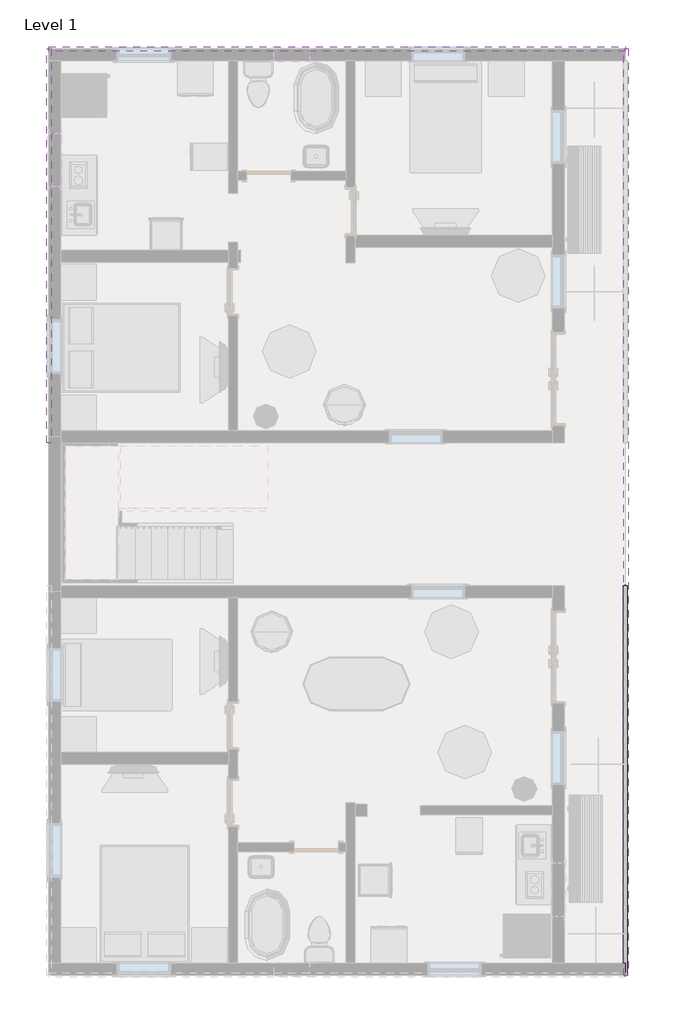
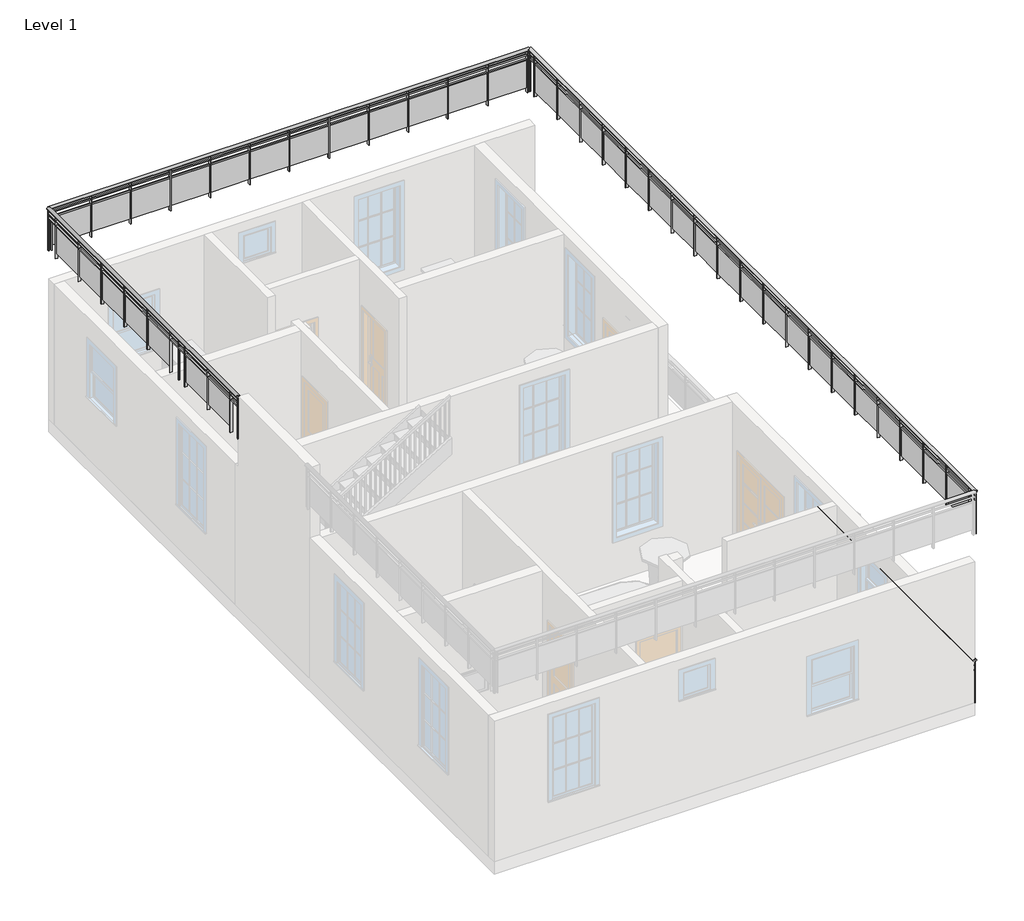
# One storey, part 3 of 4: 4 railings.
"""IFC4 building model written with IfcOpenShell, lengths in millimetres."""

from ifc_helpers import new_model, si_unit, point, frame, origin, origin_with_axes, place, context, project, spatial, polyline, ellipse_curve, trimmed, outline, extrude, element, save
from ifc_brep_helpers import plane_surface, extruded_surface, advanced_brep

model = new_model("IFC4")

# Units and contexts
model_context = context("Model", 3, world=origin())
ifc_project = project(units=[si_unit("LENGTHUNIT", "METRE", prefix="MILLI")], contexts=[model_context])

# Site, building, storey
site = spatial("IfcSite", under=ifc_project)
building = spatial("IfcBuilding", under=site)
storey = spatial("IfcBuildingStorey", under=building, Name="Level 1", Elevation=0.0)

# Railings
placement = place(None, origin())
element("IfcRailing", 1, ObjectType="Glass Panel - Bottom Fill", at=placement, inside=storey, context=model_context, shape_type="SolidModel", body=[
    advanced_brep(
    [(-4753.1750862, -655.7379829, 914.4), (-4676.9750862, -655.7379829, 914.4), (-4753.1750862, 5999.0620171, 914.4), (-4676.9750862, 5999.0620171, 914.4)],
    [
        (0, 1, ellipse_curve(frame((-4715.0750862, -655.7379829, 914.4), z_axis=(0.0, -1.0, 0.0), x_axis=(1.0, 0.0, 0.0)), 38.1, 28.575)),
        (1, 0, ellipse_curve(frame((-4715.0750862, -655.7379829, 914.4), z_axis=(0.0, -1.0, 0.0), x_axis=(1.0, 0.0, 0.0)), 38.1, 28.575)),
        (2, 3, ellipse_curve(frame((-4715.0750862, 5999.0620171, 914.4), z_axis=(0.0, 1.0, 0.0), x_axis=(1.0, 0.0, 0.0)), 38.1, 28.575)),
        (3, 2, ellipse_curve(frame((-4715.0750862, 5999.0620171, 914.4), z_axis=(0.0, 1.0, 0.0), x_axis=(1.0, 0.0, 0.0)), 38.1, 28.575)),
        (0, 2),
        (3, 1),
    ],
    [
        plane_surface(frame((-4715.0750862, -655.7379829, 914.4), z_axis=(0.0, -1.0, 0.0), x_axis=(0.0, 0.0, 1.0))),
        plane_surface(frame((-4715.0750862, 5999.0620171, 914.4), z_axis=(0.0, 1.0, 0.0), x_axis=(0.0, 0.0, 1.0))),
        extruded_surface(trimmed(ellipse_curve(frame((-4715.0750862, 5999.0620171, 914.4), z_axis=(0.0, -1.0, 0.0), x_axis=(1.0, 0.0, 0.0)), 38.1, 28.575), [point((-4753.1750862, 5999.0620171, 914.4))], [point((-4676.9750862, 5999.0620171, 914.4))], True, "CARTESIAN"), (0.0, -6654.8, 0.0), 6654.8),
        extruded_surface(trimmed(ellipse_curve(frame((-4715.0750862, 5999.0620171, 914.4), z_axis=(0.0, -1.0, 0.0), x_axis=(1.0, 0.0, 0.0)), 38.1, 28.575), [point((-4676.9750862, 5999.0620171, 914.4))], [point((-4753.1750862, 5999.0620171, 914.4))], True, "CARTESIAN"), (0.0, -6654.8, 0.0), 6654.8),
    ],
    [
        (0, [[1, 2]]),
        (1, [[3, 4]]),
        (2, [[-1, 5, -4, 6]]),
        (3, [[-2, -6, -3, -5]]),
    ],
),
    extrude(outline(polyline([(-4702.3750862, -655.7379829), (-4727.7750862, -655.7379829), (-4727.7750862, 5999.0620171), (-4702.3750862, 5999.0620171), (-4702.3750862, -655.7379829)])), frame((0.0, 0.0, 800.1), z_axis=(0.0, 0.0, 1.0), x_axis=(1.0, 0.0, 0.0)), (0.0, 0.0, 1.0), 25.4),
    extrude(outline(polyline([(-4702.3750862, -655.7379829), (-4727.7750862, -655.7379829), (-4727.7750862, 5999.0620171), (-4702.3750862, 5999.0620171), (-4702.3750862, -655.7379829)])), frame((0.0, 0.0, 698.5), z_axis=(0.0, 0.0, 1.0), x_axis=(1.0, 0.0, 0.0)), (0.0, 0.0, 1.0), 25.4),
    extrude(outline(polyline([(-4689.6750862, 5916.5120171), (-4740.4750862, 5916.5120171), (-4740.4750862, 5929.2120171), (-4689.6750862, 5929.2120171), (-4689.6750862, 5916.5120171)])), origin_with_axes(), (0.0, 0.0, 1.0), 885.6788223),
    extrude(outline(polyline([(-4721.6102432, 5110.0620171), (-4721.6102432, 5922.8620171), (-4715.2602432, 5922.8620171), (-4715.2602432, 5110.0620171), (-4721.6102432, 5110.0620171)])), frame((0.0, 0.0, 101.6), z_axis=(0.0, 0.0, 1.0), x_axis=(1.0, 0.0, 0.0)), (0.0, 0.0, 1.0), 596.9),
    extrude(outline(polyline([(-4689.6750862, 5103.7120171), (-4740.4750862, 5103.7120171), (-4740.4750862, 5116.4120171), (-4689.6750862, 5116.4120171), (-4689.6750862, 5103.7120171)])), origin_with_axes(), (0.0, 0.0, 1.0), 885.6788223),
    extrude(outline(polyline([(-4721.6102432, 4297.2620171), (-4721.6102432, 5110.0620171), (-4715.2602432, 5110.0620171), (-4715.2602432, 4297.2620171), (-4721.6102432, 4297.2620171)])), frame((0.0, 0.0, 101.6), z_axis=(0.0, 0.0, 1.0), x_axis=(1.0, 0.0, 0.0)), (0.0, 0.0, 1.0), 596.9),
    extrude(outline(polyline([(-4689.6750862, 4290.9120171), (-4740.4750862, 4290.9120171), (-4740.4750862, 4303.6120171), (-4689.6750862, 4303.6120171), (-4689.6750862, 4290.9120171)])), origin_with_axes(), (0.0, 0.0, 1.0), 885.6788223),
    extrude(outline(polyline([(-4721.6102432, 3484.4620171), (-4721.6102432, 4297.2620171), (-4715.2602432, 4297.2620171), (-4715.2602432, 3484.4620171), (-4721.6102432, 3484.4620171)])), frame((0.0, 0.0, 101.6), z_axis=(0.0, 0.0, 1.0), x_axis=(1.0, 0.0, 0.0)), (0.0, 0.0, 1.0), 596.9),
    extrude(outline(polyline([(-4689.6750862, 3478.1120171), (-4740.4750862, 3478.1120171), (-4740.4750862, 3490.8120171), (-4689.6750862, 3490.8120171), (-4689.6750862, 3478.1120171)])), origin_with_axes(), (0.0, 0.0, 1.0), 885.6788223),
    extrude(outline(polyline([(-4721.6102432, 2671.6620171), (-4721.6102432, 3484.4620171), (-4715.2602432, 3484.4620171), (-4715.2602432, 2671.6620171), (-4721.6102432, 2671.6620171)])), frame((0.0, 0.0, 101.6), z_axis=(0.0, 0.0, 1.0), x_axis=(1.0, 0.0, 0.0)), (0.0, 0.0, 1.0), 596.9),
    extrude(outline(polyline([(-4689.6750862, 2665.3120171), (-4740.4750862, 2665.3120171), (-4740.4750862, 2678.0120171), (-4689.6750862, 2678.0120171), (-4689.6750862, 2665.3120171)])), origin_with_axes(), (0.0, 0.0, 1.0), 885.6788223),
    extrude(outline(polyline([(-4721.6102432, 1858.8620171), (-4721.6102432, 2671.6620171), (-4715.2602432, 2671.6620171), (-4715.2602432, 1858.8620171), (-4721.6102432, 1858.8620171)])), frame((0.0, 0.0, 101.6), z_axis=(0.0, 0.0, 1.0), x_axis=(1.0, 0.0, 0.0)), (0.0, 0.0, 1.0), 596.9),
    extrude(outline(polyline([(-4689.6750862, 1852.5120171), (-4740.4750862, 1852.5120171), (-4740.4750862, 1865.2120171), (-4689.6750862, 1865.2120171), (-4689.6750862, 1852.5120171)])), origin_with_axes(), (0.0, 0.0, 1.0), 885.6788223),
    extrude(outline(polyline([(-4721.6102432, 1046.0620171), (-4721.6102432, 1858.8620171), (-4715.2602432, 1858.8620171), (-4715.2602432, 1046.0620171), (-4721.6102432, 1046.0620171)])), frame((0.0, 0.0, 101.6), z_axis=(0.0, 0.0, 1.0), x_axis=(1.0, 0.0, 0.0)), (0.0, 0.0, 1.0), 596.9),
    extrude(outline(polyline([(-4689.6750862, 1039.7120171), (-4740.4750862, 1039.7120171), (-4740.4750862, 1052.4120171), (-4689.6750862, 1052.4120171), (-4689.6750862, 1039.7120171)])), origin_with_axes(), (0.0, 0.0, 1.0), 885.6788223),
    extrude(outline(polyline([(-4721.6102432, 233.2620171), (-4721.6102432, 1046.0620171), (-4715.2602432, 1046.0620171), (-4715.2602432, 233.2620171), (-4721.6102432, 233.2620171)])), frame((0.0, 0.0, 101.6), z_axis=(0.0, 0.0, 1.0), x_axis=(1.0, 0.0, 0.0)), (0.0, 0.0, 1.0), 596.9),
    extrude(outline(polyline([(-4689.6750862, 226.9120171), (-4740.4750862, 226.9120171), (-4740.4750862, 239.6120171), (-4689.6750862, 239.6120171), (-4689.6750862, 226.9120171)])), origin_with_axes(), (0.0, 0.0, 1.0), 885.6788223),
    extrude(outline(polyline([(-4721.6102432, -579.5379829), (-4721.6102432, 233.2620171), (-4715.2602432, 233.2620171), (-4715.2602432, -579.5379829), (-4721.6102432, -579.5379829)])), frame((0.0, 0.0, 101.6), z_axis=(0.0, 0.0, 1.0), x_axis=(1.0, 0.0, 0.0)), (0.0, 0.0, 1.0), 596.9),
    extrude(outline(polyline([(-4689.6750862, -585.8879829), (-4740.4750862, -585.8879829), (-4740.4750862, -573.1879829), (-4689.6750862, -573.1879829), (-4689.6750862, -585.8879829)])), origin_with_axes(), (0.0, 0.0, 1.0), 885.6788223),
    extrude(outline(polyline([(-4705.5500862, 5986.3620171), (-4724.6000862, 5986.3620171), (-4724.6000862, 6005.4120171), (-4705.5500862, 6005.4120171), (-4705.5500862, 5986.3620171)])), origin_with_axes(), (0.0, 0.0, 1.0), 885.6788223),
    extrude(outline(polyline([(-4705.5500862, -662.0879829), (-4724.6000862, -662.0879829), (-4724.6000862, -643.0379829), (-4705.5500862, -643.0379829), (-4705.5500862, -662.0879829)])), origin_with_axes(), (0.0, 0.0, 1.0), 885.6788223),
])
element("IfcRailing", 2, ObjectType="Glass Panel - Bottom Fill", at=placement, inside=storey, context=model_context, shape_type="SolidModel", body=[
    advanced_brep(
    [(-4740.4750862, -655.7379829, 4572.0), (-4664.2750862, -655.7379829, 4572.0), (-4740.4750862, 15168.4620171, 4572.0), (-4664.2750862, 15168.4620171, 4572.0)],
    [
        (0, 1, ellipse_curve(frame((-4702.3750862, -655.7379829, 4572.0), z_axis=(0.0, -1.0, 0.0), x_axis=(1.0, 0.0, 0.0)), 38.1, 28.575)),
        (1, 0, ellipse_curve(frame((-4702.3750862, -655.7379829, 4572.0), z_axis=(0.0, -1.0, 0.0), x_axis=(1.0, 0.0, 0.0)), 38.1, 28.575)),
        (2, 3, ellipse_curve(frame((-4702.3750862, 15168.4620171, 4572.0), z_axis=(0.0, 1.0, 0.0), x_axis=(1.0, 0.0, 0.0)), 38.1, 28.575)),
        (3, 2, ellipse_curve(frame((-4702.3750862, 15168.4620171, 4572.0), z_axis=(0.0, 1.0, 0.0), x_axis=(1.0, 0.0, 0.0)), 38.1, 28.575)),
        (0, 2),
        (3, 1),
    ],
    [
        plane_surface(frame((-4702.3750862, -655.7379829, 4572.0), z_axis=(0.0, -1.0, 0.0), x_axis=(0.0, 0.0, 1.0))),
        plane_surface(frame((-4702.3750862, 15168.4620171, 4572.0), z_axis=(0.0, 1.0, 0.0), x_axis=(0.0, 0.0, 1.0))),
        extruded_surface(trimmed(ellipse_curve(frame((-4702.3750862, 15168.4620171, 4572.0), z_axis=(0.0, -1.0, 0.0), x_axis=(1.0, 0.0, 0.0)), 38.1, 28.575), [point((-4740.4750862, 15168.4620171, 4572.0))], [point((-4664.2750862, 15168.4620171, 4572.0))], True, "CARTESIAN"), (0.0, -15824.2, 0.0), 15824.2),
        extruded_surface(trimmed(ellipse_curve(frame((-4702.3750862, 15168.4620171, 4572.0), z_axis=(0.0, -1.0, 0.0), x_axis=(1.0, 0.0, 0.0)), 38.1, 28.575), [point((-4664.2750862, 15168.4620171, 4572.0))], [point((-4740.4750862, 15168.4620171, 4572.0))], True, "CARTESIAN"), (0.0, -15824.2, 0.0), 15824.2),
    ],
    [
        (0, [[1, 2]]),
        (1, [[3, 4]]),
        (2, [[-1, 5, -4, 6]]),
        (3, [[-2, -6, -3, -5]]),
    ],
),
    extrude(outline(polyline([(-4689.6750862, -655.7379829), (-4715.0750862, -655.7379829), (-4715.0750862, 15168.4620171), (-4689.6750862, 15168.4620171), (-4689.6750862, -655.7379829)])), frame((0.0, 0.0, 4457.7), z_axis=(0.0, 0.0, 1.0), x_axis=(1.0, 0.0, 0.0)), (0.0, 0.0, 1.0), 25.4),
    extrude(outline(polyline([(-4689.6750862, -655.7379829), (-4715.0750862, -655.7379829), (-4715.0750862, 15168.4620171), (-4689.6750862, 15168.4620171), (-4689.6750862, -655.7379829)])), frame((0.0, 0.0, 4356.1), z_axis=(0.0, 0.0, 1.0), x_axis=(1.0, 0.0, 0.0)), (0.0, 0.0, 1.0), 25.4),
    extrude(outline(polyline([(-4676.9750862, 14971.6120171), (-4727.7750862, 14971.6120171), (-4727.7750862, 14984.3120171), (-4676.9750862, 14984.3120171), (-4676.9750862, 14971.6120171)])), frame((0.0, 0.0, 3657.6), z_axis=(0.0, 0.0, 1.0), x_axis=(1.0, 0.0, 0.0)), (0.0, 0.0, 1.0), 885.6788223),
    extrude(outline(polyline([(-4708.9102432, 14165.1620171), (-4708.9102432, 14977.9620171), (-4702.5602432, 14977.9620171), (-4702.5602432, 14165.1620171), (-4708.9102432, 14165.1620171)])), frame((0.0, 0.0, 3759.2), z_axis=(0.0, 0.0, 1.0), x_axis=(1.0, 0.0, 0.0)), (0.0, 0.0, 1.0), 596.9),
    extrude(outline(polyline([(-4676.9750862, 14158.8120171), (-4727.7750862, 14158.8120171), (-4727.7750862, 14171.5120171), (-4676.9750862, 14171.5120171), (-4676.9750862, 14158.8120171)])), frame((0.0, 0.0, 3657.6), z_axis=(0.0, 0.0, 1.0), x_axis=(1.0, 0.0, 0.0)), (0.0, 0.0, 1.0), 885.6788223),
    extrude(outline(polyline([(-4708.9102432, 13352.3620171), (-4708.9102432, 14165.1620171), (-4702.5602432, 14165.1620171), (-4702.5602432, 13352.3620171), (-4708.9102432, 13352.3620171)])), frame((0.0, 0.0, 3759.2), z_axis=(0.0, 0.0, 1.0), x_axis=(1.0, 0.0, 0.0)), (0.0, 0.0, 1.0), 596.9),
    extrude(outline(polyline([(-4676.9750862, 13346.0120171), (-4727.7750862, 13346.0120171), (-4727.7750862, 13358.7120171), (-4676.9750862, 13358.7120171), (-4676.9750862, 13346.0120171)])), frame((0.0, 0.0, 3657.6), z_axis=(0.0, 0.0, 1.0), x_axis=(1.0, 0.0, 0.0)), (0.0, 0.0, 1.0), 885.6788223),
    extrude(outline(polyline([(-4708.9102432, 12539.5620171), (-4708.9102432, 13352.3620171), (-4702.5602432, 13352.3620171), (-4702.5602432, 12539.5620171), (-4708.9102432, 12539.5620171)])), frame((0.0, 0.0, 3759.2), z_axis=(0.0, 0.0, 1.0), x_axis=(1.0, 0.0, 0.0)), (0.0, 0.0, 1.0), 596.9),
    extrude(outline(polyline([(-4676.9750862, 12533.2120171), (-4727.7750862, 12533.2120171), (-4727.7750862, 12545.9120171), (-4676.9750862, 12545.9120171), (-4676.9750862, 12533.2120171)])), frame((0.0, 0.0, 3657.6), z_axis=(0.0, 0.0, 1.0), x_axis=(1.0, 0.0, 0.0)), (0.0, 0.0, 1.0), 885.6788223),
    extrude(outline(polyline([(-4708.9102432, 11726.7620171), (-4708.9102432, 12539.5620171), (-4702.5602432, 12539.5620171), (-4702.5602432, 11726.7620171), (-4708.9102432, 11726.7620171)])), frame((0.0, 0.0, 3759.2), z_axis=(0.0, 0.0, 1.0), x_axis=(1.0, 0.0, 0.0)), (0.0, 0.0, 1.0), 596.9),
    extrude(outline(polyline([(-4676.9750862, 11720.4120171), (-4727.7750862, 11720.4120171), (-4727.7750862, 11733.1120171), (-4676.9750862, 11733.1120171), (-4676.9750862, 11720.4120171)])), frame((0.0, 0.0, 3657.6), z_axis=(0.0, 0.0, 1.0), x_axis=(1.0, 0.0, 0.0)), (0.0, 0.0, 1.0), 885.6788223),
    extrude(outline(polyline([(-4708.9102432, 10913.9620171), (-4708.9102432, 11726.7620171), (-4702.5602432, 11726.7620171), (-4702.5602432, 10913.9620171), (-4708.9102432, 10913.9620171)])), frame((0.0, 0.0, 3759.2), z_axis=(0.0, 0.0, 1.0), x_axis=(1.0, 0.0, 0.0)), (0.0, 0.0, 1.0), 596.9),
    extrude(outline(polyline([(-4676.9750862, 10907.6120171), (-4727.7750862, 10907.6120171), (-4727.7750862, 10920.3120171), (-4676.9750862, 10920.3120171), (-4676.9750862, 10907.6120171)])), frame((0.0, 0.0, 3657.6), z_axis=(0.0, 0.0, 1.0), x_axis=(1.0, 0.0, 0.0)), (0.0, 0.0, 1.0), 885.6788223),
    extrude(outline(polyline([(-4708.9102432, 10101.1620171), (-4708.9102432, 10913.9620171), (-4702.5602432, 10913.9620171), (-4702.5602432, 10101.1620171), (-4708.9102432, 10101.1620171)])), frame((0.0, 0.0, 3759.2), z_axis=(0.0, 0.0, 1.0), x_axis=(1.0, 0.0, 0.0)), (0.0, 0.0, 1.0), 596.9),
    extrude(outline(polyline([(-4676.9750862, 10094.8120171), (-4727.7750862, 10094.8120171), (-4727.7750862, 10107.5120171), (-4676.9750862, 10107.5120171), (-4676.9750862, 10094.8120171)])), frame((0.0, 0.0, 3657.6), z_axis=(0.0, 0.0, 1.0), x_axis=(1.0, 0.0, 0.0)), (0.0, 0.0, 1.0), 885.6788223),
    extrude(outline(polyline([(-4708.9102432, 9288.3620171), (-4708.9102432, 10101.1620171), (-4702.5602432, 10101.1620171), (-4702.5602432, 9288.3620171), (-4708.9102432, 9288.3620171)])), frame((0.0, 0.0, 3759.2), z_axis=(0.0, 0.0, 1.0), x_axis=(1.0, 0.0, 0.0)), (0.0, 0.0, 1.0), 596.9),
    extrude(outline(polyline([(-4676.9750862, 9282.0120171), (-4727.7750862, 9282.0120171), (-4727.7750862, 9294.7120171), (-4676.9750862, 9294.7120171), (-4676.9750862, 9282.0120171)])), frame((0.0, 0.0, 3657.6), z_axis=(0.0, 0.0, 1.0), x_axis=(1.0, 0.0, 0.0)), (0.0, 0.0, 1.0), 885.6788223),
    extrude(outline(polyline([(-4708.9102432, 8475.5620171), (-4708.9102432, 9288.3620171), (-4702.5602432, 9288.3620171), (-4702.5602432, 8475.5620171), (-4708.9102432, 8475.5620171)])), frame((0.0, 0.0, 3759.2), z_axis=(0.0, 0.0, 1.0), x_axis=(1.0, 0.0, 0.0)), (0.0, 0.0, 1.0), 596.9),
    extrude(outline(polyline([(-4676.9750862, 8469.2120171), (-4727.7750862, 8469.2120171), (-4727.7750862, 8481.9120171), (-4676.9750862, 8481.9120171), (-4676.9750862, 8469.2120171)])), frame((0.0, 0.0, 3657.6), z_axis=(0.0, 0.0, 1.0), x_axis=(1.0, 0.0, 0.0)), (0.0, 0.0, 1.0), 885.6788223),
    extrude(outline(polyline([(-4708.9102432, 7662.7620171), (-4708.9102432, 8475.5620171), (-4702.5602432, 8475.5620171), (-4702.5602432, 7662.7620171), (-4708.9102432, 7662.7620171)])), frame((0.0, 0.0, 3759.2), z_axis=(0.0, 0.0, 1.0), x_axis=(1.0, 0.0, 0.0)), (0.0, 0.0, 1.0), 596.9),
    extrude(outline(polyline([(-4676.9750862, 7656.4120171), (-4727.7750862, 7656.4120171), (-4727.7750862, 7669.1120171), (-4676.9750862, 7669.1120171), (-4676.9750862, 7656.4120171)])), frame((0.0, 0.0, 3657.6), z_axis=(0.0, 0.0, 1.0), x_axis=(1.0, 0.0, 0.0)), (0.0, 0.0, 1.0), 885.6788223),
    extrude(outline(polyline([(-4708.9102432, 6849.9620171), (-4708.9102432, 7662.7620171), (-4702.5602432, 7662.7620171), (-4702.5602432, 6849.9620171), (-4708.9102432, 6849.9620171)])), frame((0.0, 0.0, 3759.2), z_axis=(0.0, 0.0, 1.0), x_axis=(1.0, 0.0, 0.0)), (0.0, 0.0, 1.0), 596.9),
    extrude(outline(polyline([(-4676.9750862, 6843.6120171), (-4727.7750862, 6843.6120171), (-4727.7750862, 6856.3120171), (-4676.9750862, 6856.3120171), (-4676.9750862, 6843.6120171)])), frame((0.0, 0.0, 3657.6), z_axis=(0.0, 0.0, 1.0), x_axis=(1.0, 0.0, 0.0)), (0.0, 0.0, 1.0), 885.6788223),
    extrude(outline(polyline([(-4708.9102432, 6037.1620171), (-4708.9102432, 6849.9620171), (-4702.5602432, 6849.9620171), (-4702.5602432, 6037.1620171), (-4708.9102432, 6037.1620171)])), frame((0.0, 0.0, 3759.2), z_axis=(0.0, 0.0, 1.0), x_axis=(1.0, 0.0, 0.0)), (0.0, 0.0, 1.0), 596.9),
    extrude(outline(polyline([(-4676.9750862, 6030.8120171), (-4727.7750862, 6030.8120171), (-4727.7750862, 6043.5120171), (-4676.9750862, 6043.5120171), (-4676.9750862, 6030.8120171)])), frame((0.0, 0.0, 3657.6), z_axis=(0.0, 0.0, 1.0), x_axis=(1.0, 0.0, 0.0)), (0.0, 0.0, 1.0), 885.6788223),
    extrude(outline(polyline([(-4708.9102432, 5224.3620171), (-4708.9102432, 6037.1620171), (-4702.5602432, 6037.1620171), (-4702.5602432, 5224.3620171), (-4708.9102432, 5224.3620171)])), frame((0.0, 0.0, 3759.2), z_axis=(0.0, 0.0, 1.0), x_axis=(1.0, 0.0, 0.0)), (0.0, 0.0, 1.0), 596.9),
    extrude(outline(polyline([(-4676.9750862, 5218.0120171), (-4727.7750862, 5218.0120171), (-4727.7750862, 5230.7120171), (-4676.9750862, 5230.7120171), (-4676.9750862, 5218.0120171)])), frame((0.0, 0.0, 3657.6), z_axis=(0.0, 0.0, 1.0), x_axis=(1.0, 0.0, 0.0)), (0.0, 0.0, 1.0), 885.6788223),
    extrude(outline(polyline([(-4708.9102432, 4411.5620171), (-4708.9102432, 5224.3620171), (-4702.5602432, 5224.3620171), (-4702.5602432, 4411.5620171), (-4708.9102432, 4411.5620171)])), frame((0.0, 0.0, 3759.2), z_axis=(0.0, 0.0, 1.0), x_axis=(1.0, 0.0, 0.0)), (0.0, 0.0, 1.0), 596.9),
    extrude(outline(polyline([(-4676.9750862, 4405.2120171), (-4727.7750862, 4405.2120171), (-4727.7750862, 4417.9120171), (-4676.9750862, 4417.9120171), (-4676.9750862, 4405.2120171)])), frame((0.0, 0.0, 3657.6), z_axis=(0.0, 0.0, 1.0), x_axis=(1.0, 0.0, 0.0)), (0.0, 0.0, 1.0), 885.6788223),
    extrude(outline(polyline([(-4708.9102432, 3598.7620171), (-4708.9102432, 4411.5620171), (-4702.5602432, 4411.5620171), (-4702.5602432, 3598.7620171), (-4708.9102432, 3598.7620171)])), frame((0.0, 0.0, 3759.2), z_axis=(0.0, 0.0, 1.0), x_axis=(1.0, 0.0, 0.0)), (0.0, 0.0, 1.0), 596.9),
    extrude(outline(polyline([(-4676.9750862, 3592.4120171), (-4727.7750862, 3592.4120171), (-4727.7750862, 3605.1120171), (-4676.9750862, 3605.1120171), (-4676.9750862, 3592.4120171)])), frame((0.0, 0.0, 3657.6), z_axis=(0.0, 0.0, 1.0), x_axis=(1.0, 0.0, 0.0)), (0.0, 0.0, 1.0), 885.6788223),
    extrude(outline(polyline([(-4708.9102432, 2785.9620171), (-4708.9102432, 3598.7620171), (-4702.5602432, 3598.7620171), (-4702.5602432, 2785.9620171), (-4708.9102432, 2785.9620171)])), frame((0.0, 0.0, 3759.2), z_axis=(0.0, 0.0, 1.0), x_axis=(1.0, 0.0, 0.0)), (0.0, 0.0, 1.0), 596.9),
    extrude(outline(polyline([(-4676.9750862, 2779.6120171), (-4727.7750862, 2779.6120171), (-4727.7750862, 2792.3120171), (-4676.9750862, 2792.3120171), (-4676.9750862, 2779.6120171)])), frame((0.0, 0.0, 3657.6), z_axis=(0.0, 0.0, 1.0), x_axis=(1.0, 0.0, 0.0)), (0.0, 0.0, 1.0), 885.6788223),
    extrude(outline(polyline([(-4708.9102432, 1973.1620171), (-4708.9102432, 2785.9620171), (-4702.5602432, 2785.9620171), (-4702.5602432, 1973.1620171), (-4708.9102432, 1973.1620171)])), frame((0.0, 0.0, 3759.2), z_axis=(0.0, 0.0, 1.0), x_axis=(1.0, 0.0, 0.0)), (0.0, 0.0, 1.0), 596.9),
    extrude(outline(polyline([(-4676.9750862, 1966.8120171), (-4727.7750862, 1966.8120171), (-4727.7750862, 1979.5120171), (-4676.9750862, 1979.5120171), (-4676.9750862, 1966.8120171)])), frame((0.0, 0.0, 3657.6), z_axis=(0.0, 0.0, 1.0), x_axis=(1.0, 0.0, 0.0)), (0.0, 0.0, 1.0), 885.6788223),
    extrude(outline(polyline([(-4708.9102432, 1160.3620171), (-4708.9102432, 1973.1620171), (-4702.5602432, 1973.1620171), (-4702.5602432, 1160.3620171), (-4708.9102432, 1160.3620171)])), frame((0.0, 0.0, 3759.2), z_axis=(0.0, 0.0, 1.0), x_axis=(1.0, 0.0, 0.0)), (0.0, 0.0, 1.0), 596.9),
    extrude(outline(polyline([(-4676.9750862, 1154.0120171), (-4727.7750862, 1154.0120171), (-4727.7750862, 1166.7120171), (-4676.9750862, 1166.7120171), (-4676.9750862, 1154.0120171)])), frame((0.0, 0.0, 3657.6), z_axis=(0.0, 0.0, 1.0), x_axis=(1.0, 0.0, 0.0)), (0.0, 0.0, 1.0), 885.6788223),
    extrude(outline(polyline([(-4708.9102432, 347.5620171), (-4708.9102432, 1160.3620171), (-4702.5602432, 1160.3620171), (-4702.5602432, 347.5620171), (-4708.9102432, 347.5620171)])), frame((0.0, 0.0, 3759.2), z_axis=(0.0, 0.0, 1.0), x_axis=(1.0, 0.0, 0.0)), (0.0, 0.0, 1.0), 596.9),
    extrude(outline(polyline([(-4676.9750862, 341.2120171), (-4727.7750862, 341.2120171), (-4727.7750862, 353.9120171), (-4676.9750862, 353.9120171), (-4676.9750862, 341.2120171)])), frame((0.0, 0.0, 3657.6), z_axis=(0.0, 0.0, 1.0), x_axis=(1.0, 0.0, 0.0)), (0.0, 0.0, 1.0), 885.6788223),
    extrude(outline(polyline([(-4708.9102432, -465.2379829), (-4708.9102432, 347.5620171), (-4702.5602432, 347.5620171), (-4702.5602432, -465.2379829), (-4708.9102432, -465.2379829)])), frame((0.0, 0.0, 3759.2), z_axis=(0.0, 0.0, 1.0), x_axis=(1.0, 0.0, 0.0)), (0.0, 0.0, 1.0), 596.9),
    extrude(outline(polyline([(-4676.9750862, -471.5879829), (-4727.7750862, -471.5879829), (-4727.7750862, -458.8879829), (-4676.9750862, -458.8879829), (-4676.9750862, -471.5879829)])), frame((0.0, 0.0, 3657.6), z_axis=(0.0, 0.0, 1.0), x_axis=(1.0, 0.0, 0.0)), (0.0, 0.0, 1.0), 885.6788223),
    extrude(outline(polyline([(-4692.8500862, 15155.7620171), (-4711.9000862, 15155.7620171), (-4711.9000862, 15174.8120171), (-4692.8500862, 15174.8120171), (-4692.8500862, 15155.7620171)])), frame((0.0, 0.0, 3657.6), z_axis=(0.0, 0.0, 1.0), x_axis=(1.0, 0.0, 0.0)), (0.0, 0.0, 1.0), 885.6788223),
    extrude(outline(polyline([(-4692.8500862, -662.0879829), (-4711.9000862, -662.0879829), (-4711.9000862, -643.0379829), (-4692.8500862, -643.0379829), (-4692.8500862, -662.0879829)])), frame((0.0, 0.0, 3657.6), z_axis=(0.0, 0.0, 1.0), x_axis=(1.0, 0.0, 0.0)), (0.0, 0.0, 1.0), 885.6788223),
])
element("IfcRailing", 3, ObjectType="Glass Panel - Bottom Fill", at=placement, inside=storey, context=model_context, shape_type="SolidModel", body=[
    advanced_brep(
    [(-4715.0750862, 15130.3620171, 4572.0), (-4715.0750862, 15206.5620171, 4572.0), (-14570.2750862, 15130.3620171, 4572.0), (-14570.2750862, 15206.5620171, 4572.0)],
    [
        (0, 1, ellipse_curve(frame((-4715.0750862, 15168.4620171, 4572.0), z_axis=(1.0, 0.0, 0.0), x_axis=(0.0, 1.0, 0.0)), 38.1, 28.575)),
        (1, 0, ellipse_curve(frame((-4715.0750862, 15168.4620171, 4572.0), z_axis=(1.0, 0.0, 0.0), x_axis=(0.0, 1.0, 0.0)), 38.1, 28.575)),
        (2, 3, ellipse_curve(frame((-14570.2750862, 15168.4620171, 4572.0), z_axis=(-1.0, 0.0, 0.0), x_axis=(0.0, 1.0, 0.0)), 38.1, 28.575)),
        (3, 2, ellipse_curve(frame((-14570.2750862, 15168.4620171, 4572.0), z_axis=(-1.0, 0.0, 0.0), x_axis=(0.0, 1.0, 0.0)), 38.1, 28.575)),
        (0, 2),
        (3, 1),
    ],
    [
        plane_surface(frame((-4715.0750862, 15168.4620171, 4572.0), z_axis=(1.0, 0.0, 0.0), x_axis=(0.0, -1.0, 0.0))),
        plane_surface(frame((-14570.2750862, 15168.4620171, 4572.0), z_axis=(-1.0, 0.0, 0.0), x_axis=(0.0, -1.0, 0.0))),
        extruded_surface(trimmed(ellipse_curve(frame((-14570.2750862, 15168.4620171, 4572.0), z_axis=(1.0, 0.0, 0.0), x_axis=(0.0, 1.0, 0.0)), 38.1, 28.575), [point((-14570.2750862, 15130.3620171, 4572.0))], [point((-14570.2750862, 15206.5620171, 4572.0))], True, "CARTESIAN"), (9855.199999999999, 0.0, 0.0), 9855.199999999999),
        extruded_surface(trimmed(ellipse_curve(frame((-14570.2750862, 15168.4620171, 4572.0), z_axis=(1.0, 0.0, 0.0), x_axis=(0.0, 1.0, 0.0)), 38.1, 28.575), [point((-14570.2750862, 15206.5620171, 4572.0))], [point((-14570.2750862, 15130.3620171, 4572.0))], True, "CARTESIAN"), (9855.199999999999, 0.0, 0.0), 9855.199999999999),
    ],
    [
        (0, [[1, 2]]),
        (1, [[3, 4]]),
        (2, [[-1, 5, -4, 6]]),
        (3, [[-2, -6, -3, -5]]),
    ],
),
    extrude(outline(polyline([(-4715.0750862, 15181.1620171), (-4715.0750862, 15155.7620171), (-14570.2750862, 15155.7620171), (-14570.2750862, 15181.1620171), (-4715.0750862, 15181.1620171)])), frame((0.0, 0.0, 4457.7), z_axis=(0.0, 0.0, 1.0), x_axis=(1.0, 0.0, 0.0)), (0.0, 0.0, 1.0), 25.4),
    extrude(outline(polyline([(-4715.0750862, 15181.1620171), (-4715.0750862, 15155.7620171), (-14570.2750862, 15155.7620171), (-14570.2750862, 15181.1620171), (-4715.0750862, 15181.1620171)])), frame((0.0, 0.0, 4356.1), z_axis=(0.0, 0.0, 1.0), x_axis=(1.0, 0.0, 0.0)), (0.0, 0.0, 1.0), 25.4),
    extrude(outline(polyline([(-14513.1250862, 15193.8620171), (-14513.1250862, 15143.0620171), (-14525.8250862, 15143.0620171), (-14525.8250862, 15193.8620171), (-14513.1250862, 15193.8620171)])), frame((0.0, 0.0, 3657.6), z_axis=(0.0, 0.0, 1.0), x_axis=(1.0, 0.0, 0.0)), (0.0, 0.0, 1.0), 885.6788223),
    extrude(outline(polyline([(-13706.6750862, 15161.9268601), (-14519.4750862, 15161.9268601), (-14519.4750862, 15168.2768601), (-13706.6750862, 15168.2768601), (-13706.6750862, 15161.9268601)])), frame((0.0, 0.0, 3759.2), z_axis=(0.0, 0.0, 1.0), x_axis=(1.0, 0.0, 0.0)), (0.0, 0.0, 1.0), 596.9),
    extrude(outline(polyline([(-13700.3250862, 15193.8620171), (-13700.3250862, 15143.0620171), (-13713.0250862, 15143.0620171), (-13713.0250862, 15193.8620171), (-13700.3250862, 15193.8620171)])), frame((0.0, 0.0, 3657.6), z_axis=(0.0, 0.0, 1.0), x_axis=(1.0, 0.0, 0.0)), (0.0, 0.0, 1.0), 885.6788223),
    extrude(outline(polyline([(-12893.8750862, 15161.9268601), (-13706.6750862, 15161.9268601), (-13706.6750862, 15168.2768601), (-12893.8750862, 15168.2768601), (-12893.8750862, 15161.9268601)])), frame((0.0, 0.0, 3759.2), z_axis=(0.0, 0.0, 1.0), x_axis=(1.0, 0.0, 0.0)), (0.0, 0.0, 1.0), 596.9),
    extrude(outline(polyline([(-12887.5250862, 15193.8620171), (-12887.5250862, 15143.0620171), (-12900.2250862, 15143.0620171), (-12900.2250862, 15193.8620171), (-12887.5250862, 15193.8620171)])), frame((0.0, 0.0, 3657.6), z_axis=(0.0, 0.0, 1.0), x_axis=(1.0, 0.0, 0.0)), (0.0, 0.0, 1.0), 885.6788223),
    extrude(outline(polyline([(-12081.0750862, 15161.9268601), (-12893.8750862, 15161.9268601), (-12893.8750862, 15168.2768601), (-12081.0750862, 15168.2768601), (-12081.0750862, 15161.9268601)])), frame((0.0, 0.0, 3759.2), z_axis=(0.0, 0.0, 1.0), x_axis=(1.0, 0.0, 0.0)), (0.0, 0.0, 1.0), 596.9),
    extrude(outline(polyline([(-12074.7250862, 15193.8620171), (-12074.7250862, 15143.0620171), (-12087.4250862, 15143.0620171), (-12087.4250862, 15193.8620171), (-12074.7250862, 15193.8620171)])), frame((0.0, 0.0, 3657.6), z_axis=(0.0, 0.0, 1.0), x_axis=(1.0, 0.0, 0.0)), (0.0, 0.0, 1.0), 885.6788223),
    extrude(outline(polyline([(-11268.2750862, 15161.9268601), (-12081.0750862, 15161.9268601), (-12081.0750862, 15168.2768601), (-11268.2750862, 15168.2768601), (-11268.2750862, 15161.9268601)])), frame((0.0, 0.0, 3759.2), z_axis=(0.0, 0.0, 1.0), x_axis=(1.0, 0.0, 0.0)), (0.0, 0.0, 1.0), 596.9),
    extrude(outline(polyline([(-11261.9250862, 15193.8620171), (-11261.9250862, 15143.0620171), (-11274.6250862, 15143.0620171), (-11274.6250862, 15193.8620171), (-11261.9250862, 15193.8620171)])), frame((0.0, 0.0, 3657.6), z_axis=(0.0, 0.0, 1.0), x_axis=(1.0, 0.0, 0.0)), (0.0, 0.0, 1.0), 885.6788223),
    extrude(outline(polyline([(-10455.4750862, 15161.9268601), (-11268.2750862, 15161.9268601), (-11268.2750862, 15168.2768601), (-10455.4750862, 15168.2768601), (-10455.4750862, 15161.9268601)])), frame((0.0, 0.0, 3759.2), z_axis=(0.0, 0.0, 1.0), x_axis=(1.0, 0.0, 0.0)), (0.0, 0.0, 1.0), 596.9),
    extrude(outline(polyline([(-10449.1250862, 15193.8620171), (-10449.1250862, 15143.0620171), (-10461.8250862, 15143.0620171), (-10461.8250862, 15193.8620171), (-10449.1250862, 15193.8620171)])), frame((0.0, 0.0, 3657.6), z_axis=(0.0, 0.0, 1.0), x_axis=(1.0, 0.0, 0.0)), (0.0, 0.0, 1.0), 885.6788223),
    extrude(outline(polyline([(-9642.6750862, 15161.9268601), (-10455.4750862, 15161.9268601), (-10455.4750862, 15168.2768601), (-9642.6750862, 15168.2768601), (-9642.6750862, 15161.9268601)])), frame((0.0, 0.0, 3759.2), z_axis=(0.0, 0.0, 1.0), x_axis=(1.0, 0.0, 0.0)), (0.0, 0.0, 1.0), 596.9),
    extrude(outline(polyline([(-9636.3250862, 15193.8620171), (-9636.3250862, 15143.0620171), (-9649.0250862, 15143.0620171), (-9649.0250862, 15193.8620171), (-9636.3250862, 15193.8620171)])), frame((0.0, 0.0, 3657.6), z_axis=(0.0, 0.0, 1.0), x_axis=(1.0, 0.0, 0.0)), (0.0, 0.0, 1.0), 885.6788223),
    extrude(outline(polyline([(-8829.8750862, 15161.9268601), (-9642.6750862, 15161.9268601), (-9642.6750862, 15168.2768601), (-8829.8750862, 15168.2768601), (-8829.8750862, 15161.9268601)])), frame((0.0, 0.0, 3759.2), z_axis=(0.0, 0.0, 1.0), x_axis=(1.0, 0.0, 0.0)), (0.0, 0.0, 1.0), 596.9),
    extrude(outline(polyline([(-8823.5250862, 15193.8620171), (-8823.5250862, 15143.0620171), (-8836.2250862, 15143.0620171), (-8836.2250862, 15193.8620171), (-8823.5250862, 15193.8620171)])), frame((0.0, 0.0, 3657.6), z_axis=(0.0, 0.0, 1.0), x_axis=(1.0, 0.0, 0.0)), (0.0, 0.0, 1.0), 885.6788223),
    extrude(outline(polyline([(-8017.0750862, 15161.9268601), (-8829.8750862, 15161.9268601), (-8829.8750862, 15168.2768601), (-8017.0750862, 15168.2768601), (-8017.0750862, 15161.9268601)])), frame((0.0, 0.0, 3759.2), z_axis=(0.0, 0.0, 1.0), x_axis=(1.0, 0.0, 0.0)), (0.0, 0.0, 1.0), 596.9),
    extrude(outline(polyline([(-8010.7250862, 15193.8620171), (-8010.7250862, 15143.0620171), (-8023.4250862, 15143.0620171), (-8023.4250862, 15193.8620171), (-8010.7250862, 15193.8620171)])), frame((0.0, 0.0, 3657.6), z_axis=(0.0, 0.0, 1.0), x_axis=(1.0, 0.0, 0.0)), (0.0, 0.0, 1.0), 885.6788223),
    extrude(outline(polyline([(-7204.2750862, 15161.9268601), (-8017.0750862, 15161.9268601), (-8017.0750862, 15168.2768601), (-7204.2750862, 15168.2768601), (-7204.2750862, 15161.9268601)])), frame((0.0, 0.0, 3759.2), z_axis=(0.0, 0.0, 1.0), x_axis=(1.0, 0.0, 0.0)), (0.0, 0.0, 1.0), 596.9),
    extrude(outline(polyline([(-7197.9250862, 15193.8620171), (-7197.9250862, 15143.0620171), (-7210.6250862, 15143.0620171), (-7210.6250862, 15193.8620171), (-7197.9250862, 15193.8620171)])), frame((0.0, 0.0, 3657.6), z_axis=(0.0, 0.0, 1.0), x_axis=(1.0, 0.0, 0.0)), (0.0, 0.0, 1.0), 885.6788223),
    extrude(outline(polyline([(-6391.4750862, 15161.9268601), (-7204.2750862, 15161.9268601), (-7204.2750862, 15168.2768601), (-6391.4750862, 15168.2768601), (-6391.4750862, 15161.9268601)])), frame((0.0, 0.0, 3759.2), z_axis=(0.0, 0.0, 1.0), x_axis=(1.0, 0.0, 0.0)), (0.0, 0.0, 1.0), 596.9),
    extrude(outline(polyline([(-6385.1250862, 15193.8620171), (-6385.1250862, 15143.0620171), (-6397.8250862, 15143.0620171), (-6397.8250862, 15193.8620171), (-6385.1250862, 15193.8620171)])), frame((0.0, 0.0, 3657.6), z_axis=(0.0, 0.0, 1.0), x_axis=(1.0, 0.0, 0.0)), (0.0, 0.0, 1.0), 885.6788223),
    extrude(outline(polyline([(-5578.6750862, 15161.9268601), (-6391.4750862, 15161.9268601), (-6391.4750862, 15168.2768601), (-5578.6750862, 15168.2768601), (-5578.6750862, 15161.9268601)])), frame((0.0, 0.0, 3759.2), z_axis=(0.0, 0.0, 1.0), x_axis=(1.0, 0.0, 0.0)), (0.0, 0.0, 1.0), 596.9),
    extrude(outline(polyline([(-5572.3250862, 15193.8620171), (-5572.3250862, 15143.0620171), (-5585.0250862, 15143.0620171), (-5585.0250862, 15193.8620171), (-5572.3250862, 15193.8620171)])), frame((0.0, 0.0, 3657.6), z_axis=(0.0, 0.0, 1.0), x_axis=(1.0, 0.0, 0.0)), (0.0, 0.0, 1.0), 885.6788223),
    extrude(outline(polyline([(-4765.8750862, 15161.9268601), (-5578.6750862, 15161.9268601), (-5578.6750862, 15168.2768601), (-4765.8750862, 15168.2768601), (-4765.8750862, 15161.9268601)])), frame((0.0, 0.0, 3759.2), z_axis=(0.0, 0.0, 1.0), x_axis=(1.0, 0.0, 0.0)), (0.0, 0.0, 1.0), 596.9),
    extrude(outline(polyline([(-4759.5250862, 15193.8620171), (-4759.5250862, 15143.0620171), (-4772.2250862, 15143.0620171), (-4772.2250862, 15193.8620171), (-4759.5250862, 15193.8620171)])), frame((0.0, 0.0, 3657.6), z_axis=(0.0, 0.0, 1.0), x_axis=(1.0, 0.0, 0.0)), (0.0, 0.0, 1.0), 885.6788223),
    extrude(outline(polyline([(-14557.5750862, 15177.9870171), (-14557.5750862, 15158.9370171), (-14576.6250862, 15158.9370171), (-14576.6250862, 15177.9870171), (-14557.5750862, 15177.9870171)])), frame((0.0, 0.0, 3657.6), z_axis=(0.0, 0.0, 1.0), x_axis=(1.0, 0.0, 0.0)), (0.0, 0.0, 1.0), 885.6788223),
    extrude(outline(polyline([(-4708.7250862, 15177.9870171), (-4708.7250862, 15158.9370171), (-4727.7750862, 15158.9370171), (-4727.7750862, 15177.9870171), (-4708.7250862, 15177.9870171)])), frame((0.0, 0.0, 3657.6), z_axis=(0.0, 0.0, 1.0), x_axis=(1.0, 0.0, 0.0)), (0.0, 0.0, 1.0), 885.6788223),
])
element("IfcRailing", 4, ObjectType="Glass Panel - Bottom Fill", at=placement, inside=storey, context=model_context, shape_type="SolidModel", body=[
    advanced_brep(
    [(-14532.1750862, 15168.4620171, 4572.0), (-14608.3750862, 15168.4620171, 4572.0), (-14532.1750862, 8437.4620171, 4572.0), (-14608.3750862, 8437.4620171, 4572.0)],
    [
        (0, 1, ellipse_curve(frame((-14570.2750862, 15168.4620171, 4572.0), z_axis=(0.0, 1.0, 0.0), x_axis=(-1.0, 0.0, 0.0)), 38.1, 28.575)),
        (1, 0, ellipse_curve(frame((-14570.2750862, 15168.4620171, 4572.0), z_axis=(0.0, 1.0, 0.0), x_axis=(-1.0, 0.0, 0.0)), 38.1, 28.575)),
        (2, 3, ellipse_curve(frame((-14570.2750862, 8437.4620171, 4572.0), z_axis=(0.0, -1.0, 0.0), x_axis=(-1.0, 0.0, 0.0)), 38.1, 28.575)),
        (3, 2, ellipse_curve(frame((-14570.2750862, 8437.4620171, 4572.0), z_axis=(0.0, -1.0, 0.0), x_axis=(-1.0, 0.0, 0.0)), 38.1, 28.575)),
        (0, 2),
        (3, 1),
    ],
    [
        plane_surface(frame((-14570.2750862, 15168.4620171, 4572.0), z_axis=(0.0, 1.0, 0.0), x_axis=(0.0, 0.0, -1.0))),
        plane_surface(frame((-14570.2750862, 8437.4620171, 4572.0), z_axis=(0.0, -1.0, 0.0), x_axis=(0.0, 0.0, -1.0))),
        extruded_surface(trimmed(ellipse_curve(frame((-14570.2750862, 8437.4620171, 4572.0), z_axis=(0.0, 1.0, 0.0), x_axis=(-1.0, 0.0, 0.0)), 38.1, 28.575), [point((-14532.1750862, 8437.4620171, 4572.0))], [point((-14608.3750862, 8437.4620171, 4572.0))], True, "CARTESIAN"), (0.0, 6731.0, 0.0), 6731.0),
        extruded_surface(trimmed(ellipse_curve(frame((-14570.2750862, 8437.4620171, 4572.0), z_axis=(0.0, 1.0, 0.0), x_axis=(-1.0, 0.0, 0.0)), 38.1, 28.575), [point((-14608.3750862, 8437.4620171, 4572.0))], [point((-14532.1750862, 8437.4620171, 4572.0))], True, "CARTESIAN"), (0.0, 6731.0, 0.0), 6731.0),
    ],
    [
        (0, [[1, 2]]),
        (1, [[3, 4]]),
        (2, [[-1, 5, -4, 6]]),
        (3, [[-2, -6, -3, -5]]),
    ],
),
    extrude(outline(polyline([(-14582.9750862, 15168.4620171), (-14557.5750862, 15168.4620171), (-14557.5750862, 8437.4620171), (-14582.9750862, 8437.4620171), (-14582.9750862, 15168.4620171)])), frame((0.0, 0.0, 4457.7), z_axis=(0.0, 0.0, 1.0), x_axis=(1.0, 0.0, 0.0)), (0.0, 0.0, 1.0), 25.4),
    extrude(outline(polyline([(-14582.9750862, 15168.4620171), (-14557.5750862, 15168.4620171), (-14557.5750862, 8437.4620171), (-14582.9750862, 8437.4620171), (-14582.9750862, 15168.4620171)])), frame((0.0, 0.0, 4356.1), z_axis=(0.0, 0.0, 1.0), x_axis=(1.0, 0.0, 0.0)), (0.0, 0.0, 1.0), 25.4),
    extrude(outline(polyline([(-14595.6750862, 8681.9370171), (-14544.8750862, 8681.9370171), (-14544.8750862, 8669.2370171), (-14595.6750862, 8669.2370171), (-14595.6750862, 8681.9370171)])), frame((0.0, 0.0, 3657.6), z_axis=(0.0, 0.0, 1.0), x_axis=(1.0, 0.0, 0.0)), (0.0, 0.0, 1.0), 885.6788223),
    extrude(outline(polyline([(-14563.7399292, 9488.3870171), (-14563.7399292, 8675.5870171), (-14570.0899292, 8675.5870171), (-14570.0899292, 9488.3870171), (-14563.7399292, 9488.3870171)])), frame((0.0, 0.0, 3759.2), z_axis=(0.0, 0.0, 1.0), x_axis=(1.0, 0.0, 0.0)), (0.0, 0.0, 1.0), 596.9),
    extrude(outline(polyline([(-14595.6750862, 9494.7370171), (-14544.8750862, 9494.7370171), (-14544.8750862, 9482.0370171), (-14595.6750862, 9482.0370171), (-14595.6750862, 9494.7370171)])), frame((0.0, 0.0, 3657.6), z_axis=(0.0, 0.0, 1.0), x_axis=(1.0, 0.0, 0.0)), (0.0, 0.0, 1.0), 885.6788223),
    extrude(outline(polyline([(-14563.7399292, 10301.1870171), (-14563.7399292, 9488.3870171), (-14570.0899292, 9488.3870171), (-14570.0899292, 10301.1870171), (-14563.7399292, 10301.1870171)])), frame((0.0, 0.0, 3759.2), z_axis=(0.0, 0.0, 1.0), x_axis=(1.0, 0.0, 0.0)), (0.0, 0.0, 1.0), 596.9),
    extrude(outline(polyline([(-14595.6750862, 10307.5370171), (-14544.8750862, 10307.5370171), (-14544.8750862, 10294.8370171), (-14595.6750862, 10294.8370171), (-14595.6750862, 10307.5370171)])), frame((0.0, 0.0, 3657.6), z_axis=(0.0, 0.0, 1.0), x_axis=(1.0, 0.0, 0.0)), (0.0, 0.0, 1.0), 885.6788223),
    extrude(outline(polyline([(-14595.6750862, 10828.2370171), (-14544.8750862, 10828.2370171), (-14544.8750862, 10815.5370171), (-14595.6750862, 10815.5370171), (-14595.6750862, 10828.2370171)])), frame((0.0, 0.0, 3657.6), z_axis=(0.0, 0.0, 1.0), x_axis=(1.0, 0.0, 0.0)), (0.0, 0.0, 1.0), 885.6788223),
    extrude(outline(polyline([(-14563.7399292, 11634.6870171), (-14563.7399292, 10821.8870171), (-14570.0899292, 10821.8870171), (-14570.0899292, 11634.6870171), (-14563.7399292, 11634.6870171)])), frame((0.0, 0.0, 3759.2), z_axis=(0.0, 0.0, 1.0), x_axis=(1.0, 0.0, 0.0)), (0.0, 0.0, 1.0), 596.9),
    extrude(outline(polyline([(-14595.6750862, 11641.0370171), (-14544.8750862, 11641.0370171), (-14544.8750862, 11628.3370171), (-14595.6750862, 11628.3370171), (-14595.6750862, 11641.0370171)])), frame((0.0, 0.0, 3657.6), z_axis=(0.0, 0.0, 1.0), x_axis=(1.0, 0.0, 0.0)), (0.0, 0.0, 1.0), 885.6788223),
    extrude(outline(polyline([(-14563.7399292, 12447.4870171), (-14563.7399292, 11634.6870171), (-14570.0899292, 11634.6870171), (-14570.0899292, 12447.4870171), (-14563.7399292, 12447.4870171)])), frame((0.0, 0.0, 3759.2), z_axis=(0.0, 0.0, 1.0), x_axis=(1.0, 0.0, 0.0)), (0.0, 0.0, 1.0), 596.9),
    extrude(outline(polyline([(-14595.6750862, 12453.8370171), (-14544.8750862, 12453.8370171), (-14544.8750862, 12441.1370171), (-14595.6750862, 12441.1370171), (-14595.6750862, 12453.8370171)])), frame((0.0, 0.0, 3657.6), z_axis=(0.0, 0.0, 1.0), x_axis=(1.0, 0.0, 0.0)), (0.0, 0.0, 1.0), 885.6788223),
    extrude(outline(polyline([(-14563.7399292, 13260.2870171), (-14563.7399292, 12447.4870171), (-14570.0899292, 12447.4870171), (-14570.0899292, 13260.2870171), (-14563.7399292, 13260.2870171)])), frame((0.0, 0.0, 3759.2), z_axis=(0.0, 0.0, 1.0), x_axis=(1.0, 0.0, 0.0)), (0.0, 0.0, 1.0), 596.9),
    extrude(outline(polyline([(-14595.6750862, 13266.6370171), (-14544.8750862, 13266.6370171), (-14544.8750862, 13253.9370171), (-14595.6750862, 13253.9370171), (-14595.6750862, 13266.6370171)])), frame((0.0, 0.0, 3657.6), z_axis=(0.0, 0.0, 1.0), x_axis=(1.0, 0.0, 0.0)), (0.0, 0.0, 1.0), 885.6788223),
    extrude(outline(polyline([(-14563.7399292, 14073.0870171), (-14563.7399292, 13260.2870171), (-14570.0899292, 13260.2870171), (-14570.0899292, 14073.0870171), (-14563.7399292, 14073.0870171)])), frame((0.0, 0.0, 3759.2), z_axis=(0.0, 0.0, 1.0), x_axis=(1.0, 0.0, 0.0)), (0.0, 0.0, 1.0), 596.9),
    extrude(outline(polyline([(-14595.6750862, 14079.4370171), (-14544.8750862, 14079.4370171), (-14544.8750862, 14066.7370171), (-14595.6750862, 14066.7370171), (-14595.6750862, 14079.4370171)])), frame((0.0, 0.0, 3657.6), z_axis=(0.0, 0.0, 1.0), x_axis=(1.0, 0.0, 0.0)), (0.0, 0.0, 1.0), 885.6788223),
    extrude(outline(polyline([(-14563.7399292, 14885.8870171), (-14563.7399292, 14073.0870171), (-14570.0899292, 14073.0870171), (-14570.0899292, 14885.8870171), (-14563.7399292, 14885.8870171)])), frame((0.0, 0.0, 3759.2), z_axis=(0.0, 0.0, 1.0), x_axis=(1.0, 0.0, 0.0)), (0.0, 0.0, 1.0), 596.9),
    extrude(outline(polyline([(-14595.6750862, 14892.2370171), (-14544.8750862, 14892.2370171), (-14544.8750862, 14879.5370171), (-14595.6750862, 14879.5370171), (-14595.6750862, 14892.2370171)])), frame((0.0, 0.0, 3657.6), z_axis=(0.0, 0.0, 1.0), x_axis=(1.0, 0.0, 0.0)), (0.0, 0.0, 1.0), 885.6788223),
    extrude(outline(polyline([(-14579.8000862, 10548.8370171), (-14560.7500862, 10548.8370171), (-14560.7500862, 10529.7870171), (-14579.8000862, 10529.7870171), (-14579.8000862, 10548.8370171)])), frame((0.0, 0.0, 3657.6), z_axis=(0.0, 0.0, 1.0), x_axis=(1.0, 0.0, 0.0)), (0.0, 0.0, 1.0), 885.6788223),
    extrude(outline(polyline([(-14579.8000862, 8450.1620171), (-14560.7500862, 8450.1620171), (-14560.7500862, 8431.1120171), (-14579.8000862, 8431.1120171), (-14579.8000862, 8450.1620171)])), frame((0.0, 0.0, 3657.6), z_axis=(0.0, 0.0, 1.0), x_axis=(1.0, 0.0, 0.0)), (0.0, 0.0, 1.0), 885.6788223),
    extrude(outline(polyline([(-14579.8000862, 15174.8120171), (-14560.7500862, 15174.8120171), (-14560.7500862, 15155.7620171), (-14579.8000862, 15155.7620171), (-14579.8000862, 15174.8120171)])), frame((0.0, 0.0, 3657.6), z_axis=(0.0, 0.0, 1.0), x_axis=(1.0, 0.0, 0.0)), (0.0, 0.0, 1.0), 885.6788223),
])

save(model, "model.ifc")

# Revit data of these elements
# Type "Glass Panel - Bottom Fill"
#   Assembly Code = "C2010400"
#   built-in parameter 1008612 = 0.0416667 (stored number, unit not read)
#   built-in parameter 1008611 = 0.0416667 (stored number, unit not read)
#   built-in parameter 1008609 = 0.333333 (stored number, unit not read)
#   built-in parameter 1008604 = 0.166667 (stored number, unit not read)
#   built-in parameter 1008603 = 0.166667 (stored number, unit not read)
#   Railing Height = 3' - 0"
#   built-in parameter 1008630 = 2
#   built-in parameter 1008610 = 2
#   built-in parameter 1008618 = Baluster - Square : 3/4"
# Element 1 (IfcRailing, "Glass Panel - Bottom Fill")
#   Phase Created = New Construction
#   Materials on its faces: "Glass"
# Elements 2, 3, 4 (IfcRailing, "Glass Panel - Bottom Fill")
#   built-in parameter 1008621 = 12 (stored number, unit not read)
#   Phase Created = New Construction
#   Materials on its faces: "Glass"
# Materials
#   "Glass": class "Glass", colour RGB 0 128 192, transparency 0.75, Description = "Soda Lime Glass", Cost = 0
